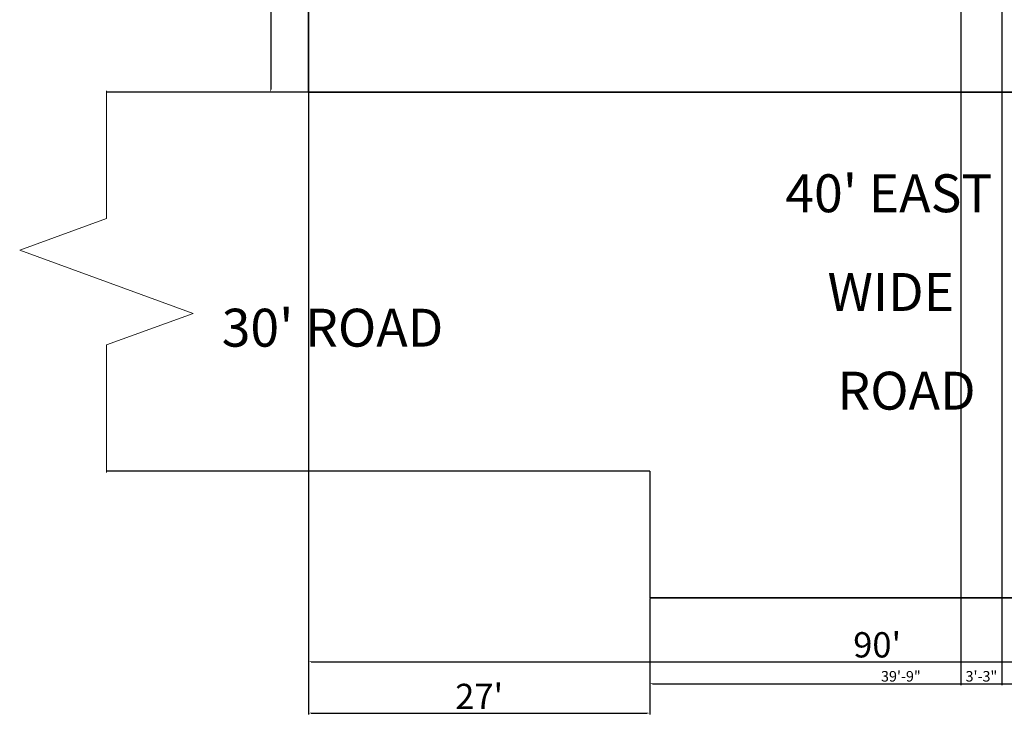
# Model space of a CAD drawing. Units: inches. Extents: x 2214 to 3937, y 762 to 2085.
# Tile 1 of 9: x 2308 to 3243, y 763 to 1424. Entities that reach past the tile are written whole.
import ezdxf

# ---------------------------------------------------------------- set-up
doc = ezdxf.new("R2010")
doc.units = ezdxf.units.IN
for name, color, linetype, lineweight in [('C-ANNO-DIMS', 2, 'Continuous', 18), ('C-ANNO-TEXT', 2, 'Continuous', 25), ('C-PROP', 3, 'Continuous', 35), ('C-ROAD', 2, 'Continuous', 25), ('C-ROAD-SYMB', 2, 'Continuous', 18)]:
    doc.layers.add(name, color=color, linetype=linetype, lineweight=lineweight)
doc.styles.get("Standard").update_dxf_attribs({"font": 'arial.ttf'})
doc.dimstyles.new('ISO-25', dxfattribs={"dimtxt": 10, "dimasz": 2.5, "dimexe": 1.25, "dimexo": 0.625, "dimtad": 1, "dimdec": 1, "dimlunit": 4, "dimtxsty": 'Standard', "dimcen": 2.5, "dimadec": 0, "dimazin": 0, "dimtfac": 1, "dimtdec": 1, "dimtmove": 0, "dimatfit": 3, "dimfxl": 1, "dimarcsym": 0})

# ---------------------------------------------------------------- blocks, each defined once
blk = doc.blocks.new('*D14')
at = {"layer": 'C-ANNO-DIMS', "color": 0, "lineweight": -2, "ltscale": 0.3, "transparency": 16777216}
for p, q in [((2582.56, 1354.59), (2582.56, 813.24)), ((3662.56, 1354.59), (3662.56, 813.24)), ((2585.06, 814.49), (3660.06, 814.49))]:
    blk.add_line(p, q, dxfattribs=at)
at = {"layer": 'C-ANNO-DIMS', "color": 0, "ltscale": 0.3, "transparency": 16777216}
for points in [[(2585.06, 814.91), (2585.06, 814.08), (2582.56, 814.49)], [(3660.06, 814.91), (3660.06, 814.08), (3662.56, 814.49)]]:
    blk.add_solid(points, dxfattribs=at)
at = {"layer": 'Defpoints', "color": 0, "ltscale": 0.3, "transparency": 16777216}
for p in [(2582.56, 1355.22), (3662.56, 1355.22), (3662.56, 814.49)]:
    blk.add_point(p, dxfattribs=at)
at = {"layer": 'C-ANNO-DIMS', "color": 0, "ltscale": 0.3, "transparency": 16777216, "insert": (3122.56, 827.37), "char_height": 24, "attachment_point": 5}
blk.add_mtext("90'", dxfattribs=at)
blk = doc.blocks.new('*D15')
at = {"layer": 'C-ANNO-DIMS', "color": 0, "lineweight": -2, "ltscale": 0.3, "transparency": 16777216}
for p, q in [((2582.56, 1354.59), (2582.56, 764.44)), ((2906.56, 874.59), (2906.56, 764.44)), ((2585.06, 765.69), (2904.06, 765.69))]:
    blk.add_line(p, q, dxfattribs=at)
at = {"layer": 'C-ANNO-DIMS', "color": 0, "ltscale": 0.3, "transparency": 16777216}
for points in [[(2585.06, 766.11), (2585.06, 765.28), (2582.56, 765.69)], [(2904.06, 766.11), (2904.06, 765.28), (2906.56, 765.69)]]:
    blk.add_solid(points, dxfattribs=at)
at = {"layer": 'Defpoints', "color": 0, "ltscale": 0.3, "transparency": 16777216}
for p in [(2582.56, 1355.22), (2906.56, 875.22), (2906.56, 765.69)]:
    blk.add_point(p, dxfattribs=at)
at = {"layer": 'C-ANNO-DIMS', "color": 0, "ltscale": 0.3, "transparency": 16777216, "insert": (2744.56, 778.37), "char_height": 24, "attachment_point": 5}
blk.add_mtext("27'", dxfattribs=at)
blk = doc.blocks.new('*D20')
at = {"layer": 'C-ANNO-DIMS', "color": 0, "lineweight": -2, "ltscale": 0.3, "transparency": 16777216}
for p, q in [((2581.93, 2003.22), (2545.31, 2003.22)), ((2546.56, 2000.72), (2546.56, 1357.72)), ((2581.93, 1355.22), (2545.31, 1355.22))]:
    blk.add_line(p, q, dxfattribs=at)
at = {"layer": 'C-ANNO-DIMS', "color": 0, "ltscale": 0.3, "transparency": 16777216}
for points in [[(2546.14, 2000.72), (2546.97, 2000.72), (2546.56, 2003.22)], [(2546.14, 1357.72), (2546.97, 1357.72), (2546.56, 1355.22)]]:
    blk.add_solid(points, dxfattribs=at)
at = {"layer": 'Defpoints', "color": 0, "ltscale": 0.3, "transparency": 16777216}
for p in [(2582.56, 2003.22), (2546.56, 1355.22), (2582.56, 1355.22)]:
    blk.add_point(p, dxfattribs=at)
at = {"layer": 'C-ANNO-DIMS', "color": 0, "ltscale": 0.3, "transparency": 16777216, "insert": (2533.73, 1679.22), "char_height": 24, "attachment_point": 5, "rotation": 90}
blk.add_mtext("54'", dxfattribs=at)
blk = doc.blocks.new('ROAD-BREAK-30FT')
at = {"ltscale": 0.3}
blk.add_lwpolyline([(82.42, 362.5), (82.42, 241.25), (0, 211.25), (164.85, 151.25), (82.42, 121.25), (82.42, 0)], dxfattribs=at)
blk = doc.blocks.new('*D61')
at = {"layer": 'C-ANNO-DIMS', "color": 0, "lineweight": -2, "ltscale": 0.3, "transparency": 16777216}
for p, q in [((2906.56, 874.59), (2906.56, 792.32)), ((3383.56, 874.59), (3383.56, 792.32)), ((2909.06, 793.57), (3381.06, 793.57))]:
    blk.add_line(p, q, dxfattribs=at)
at = {"layer": 'C-ANNO-DIMS', "color": 0, "ltscale": 0.3, "transparency": 16777216}
for points in [[(2909.06, 793.99), (2909.06, 793.15), (2906.56, 793.57)], [(3381.06, 793.99), (3381.06, 793.15), (3383.56, 793.57)]]:
    blk.add_solid(points, dxfattribs=at)
at = {"layer": 'Defpoints', "color": 0, "ltscale": 0.3, "transparency": 16777216}
for p in [(2906.56, 875.22), (3383.56, 875.22), (3383.56, 793.57)]:
    blk.add_point(p, dxfattribs=at)
at = {"layer": 'C-ANNO-DIMS', "color": 0, "ltscale": 0.3, "transparency": 16777216, "insert": (3145.06, 799.3), "char_height": 10, "attachment_point": 5}
blk.add_mtext('39\'-9"', dxfattribs=at)
blk = doc.blocks.new('*D64')
at = {"layer": 'C-ANNO-DIMS', "color": 0, "lineweight": -2, "ltscale": 0.3, "transparency": 16777216}
for p, q in [((3202.06, 1736.09), (3202.06, 792.32)), ((3241.06, 1736.09), (3241.06, 792.32)), ((3204.56, 793.57), (3238.56, 793.57))]:
    blk.add_line(p, q, dxfattribs=at)
at = {"layer": 'C-ANNO-DIMS', "color": 0, "ltscale": 0.3, "transparency": 16777216}
for points in [[(3204.56, 793.99), (3204.56, 793.15), (3202.06, 793.57)], [(3238.56, 793.99), (3238.56, 793.15), (3241.06, 793.57)]]:
    blk.add_solid(points, dxfattribs=at)
at = {"layer": 'Defpoints', "color": 0, "ltscale": 0.3, "transparency": 16777216}
for p in [(3202.06, 1736.72), (3241.06, 1736.72), (3241.06, 793.57)]:
    blk.add_point(p, dxfattribs=at)
at = {"layer": 'C-ANNO-DIMS', "color": 0, "ltscale": 0.3, "transparency": 16777216, "insert": (3221.56, 799.3), "char_height": 10, "attachment_point": 5}
blk.add_mtext('3\'-3"', dxfattribs=at)

msp = doc.modelspace()

# ---------------------------------------------------------------- linework, layer by layer
at = {"layer": 'C-PROP'}
for p, q in [((2582.56, 1355.22), (2582.56, 2003.22)), ((3662.56, 1355.22), (2582.56, 1355.22))]:
    msp.add_line(p, q, dxfattribs=at)
at = {"layer": 'C-ROAD', "ltscale": 0.3}
for p, q in [((2510.56, 1355.22), (2390.56, 1355.22)), ((2582.56, 1355.22), (2510.56, 1355.22)), ((2510.56, 995.22), (2390.56, 995.22)), ((2582.56, 995.22), (2510.56, 995.22)), ((2906.56, 995.22), (2906.56, 875.22)), ((2906.56, 875.22), (3383.56, 875.22))]:
    msp.add_line(p, q, dxfattribs=at)
at = {"layer": 'C-ROAD'}
for p, q in [((2906.56, 995.22), (2582.56, 995.22)), ((3383.56, 875.22), (2906.56, 875.22))]:
    msp.add_line(p, q, dxfattribs=at)

# ---------------------------------------------------------------- block references
at = {"layer": 'C-ROAD-SYMB', "rotation": 180}
msp.add_blockref('ROAD-BREAK-30FT', (2472.98, 1356.47), dxfattribs=at)

# ---------------------------------------------------------------- texts
at = {"layer": 'C-ANNO-TEXT', "ltscale": 0.3}
for s, p in [("40' EAST", (3035.36, 1241.23)), ('WIDE', (3075.4, 1147.51)), ("30' ROAD ", (2500.02, 1113.59)), ('ROAD', (3084.77, 1053.79))]:
    msp.add_text(s, height=36, dxfattribs=at).set_placement(p)

# ---------------------------------------------------------------- dimensions: what is measured, and where the dimension line sits
at = {"layer": 'C-ANNO-DIMS', "ltscale": 0.3}
dim = msp.add_linear_dim(base=(2546.56, 1355.22), p1=(2582.56, 2003.22), p2=(2582.56, 1355.22), angle=90, dimstyle='ISO-25', override={"dimtxt": 24, "dimclrd": 0, "dimclre": 0, "dimclrt": 0}, dxfattribs=at)
dim.commit()
dim.dimension.update_dxf_attribs({"geometry": '*D20', "text_midpoint": (2533.73, 1679.22)})
for base, p1, p2, override, picture, middle in [((3241.06, 793.57), (3202.06, 1736.72), (3241.06, 1736.72), {"dimdec": 1, "dimlfac": 1, "dimrnd": 0, "dimzin": 1, "dimdsep": 46, "dimlunit": 4, "dimfrac": 2}, '*D64', (3221.56, 799.3)), ((3662.56, 814.49), (2582.56, 1355.22), (3662.56, 1355.22), {"dimtxt": 24, "dimclrd": 0, "dimclre": 0, "dimclrt": 0}, '*D14', (3122.56, 827.37)), ((2906.56, 765.69), (2582.56, 1355.22), (2906.56, 875.22), {"dimtxt": 24, "dimclrd": 0, "dimclre": 0, "dimclrt": 0}, '*D15', (2744.56, 778.37)), ((3383.56, 793.57), (2906.56, 875.22), (3383.56, 875.22), {"dimdec": 1, "dimlfac": 1, "dimrnd": 0, "dimzin": 1, "dimdsep": 46, "dimlunit": 4, "dimfrac": 2}, '*D61', (3145.06, 799.3))]:
    dim = msp.add_linear_dim(base=base, p1=p1, p2=p2, dimstyle='ISO-25', override=override, dxfattribs=at)
    dim.commit()
    dim.dimension.update_dxf_attribs({"geometry": picture, "text_midpoint": middle})

doc.saveas('drawing.dxf')
